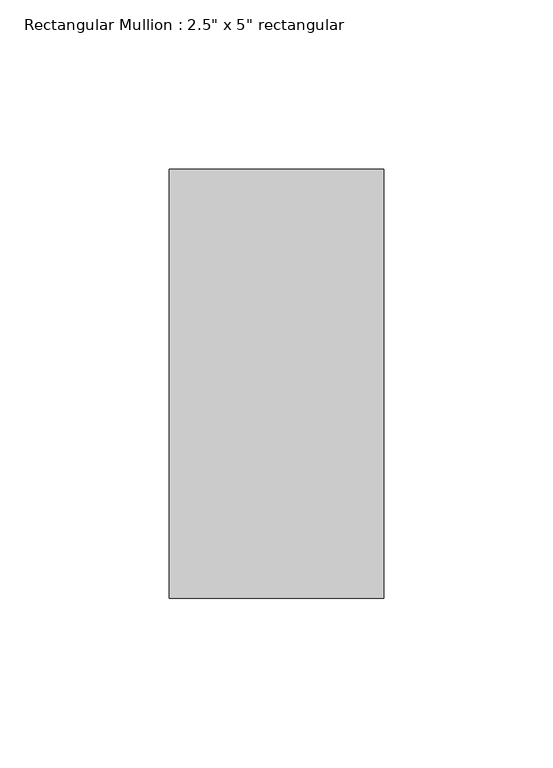
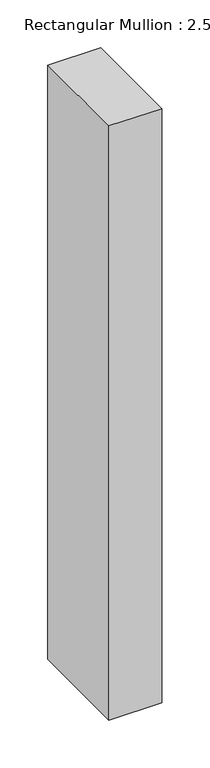
"""IFC4 building model written with IfcOpenShell, lengths in millimetres: member geometry."""

from ifc_helpers import new_model, si_unit, frame, origin, place, context, project, spatial, polyline, outline, extrude, source, transform, mapped, element, save


def member_a3a7b6e3(model_context):
    return source(origin(), model_context, "Body", "SweptSolid", [
        extrude(outline(polyline([(0.0, 63.5), (0.0, -63.5), (-63.5, -63.5), (-63.5, 63.5), (0.0, 63.5)])), frame((0.0, 0.0, -755.65), z_axis=(0.0, 0.0, 1.0), x_axis=(1.0, 0.0, 0.0)), (0.0, 0.0, 1.0), 755.65),
    ])


if __name__ == "__main__":
    model = new_model("IFC4")
    model_context = context("Model", 3, world=origin())
    ifc_project = project(units=[si_unit("LENGTHUNIT", "METRE", prefix="MILLI")], contexts=[model_context])
    site = spatial("IfcSite", under=ifc_project)
    building = spatial("IfcBuilding", under=site)
    placement = place(None, origin())
    member_shape = member_a3a7b6e3(model_context)
    element("IfcMember", 1, ObjectType="Rectangular Mullion : 2.5\" x 5\" rectangular", at=placement, inside=building, context=model_context, shape_type="MappedRepresentation", body=[
        mapped(member_shape, transform((0.0, 0.0, 0.0), x_axis=(1.0, 0.0, 0.0), y_axis=(0.0, 1.0, 0.0), z_axis=(0.0, 0.0, 1.0))),
    ])
    save(model, "model.ifc")

# Revit data of these elements
# Type "Rectangular Mullion : 2.5\" x 5\" rectangular"
#   built-in parameter 1007304 = 0.416667 (stored number, unit not read)
#   built-in parameter 1007301 = 0.104167 (stored number, unit not read)
#   built-in parameter 1007300 = 0.104167 (stored number, unit not read)
# Element 1 (IfcMember, "Rectangular Mullion : 2.5\" x 5\" rectangular")
#   Materials on its faces: "Aluminum"
# Materials
#   "Aluminum": class "Metal", colour RGB 247 247 247, transparency 0, Description = "Aluminum 6061", Cost = 0
